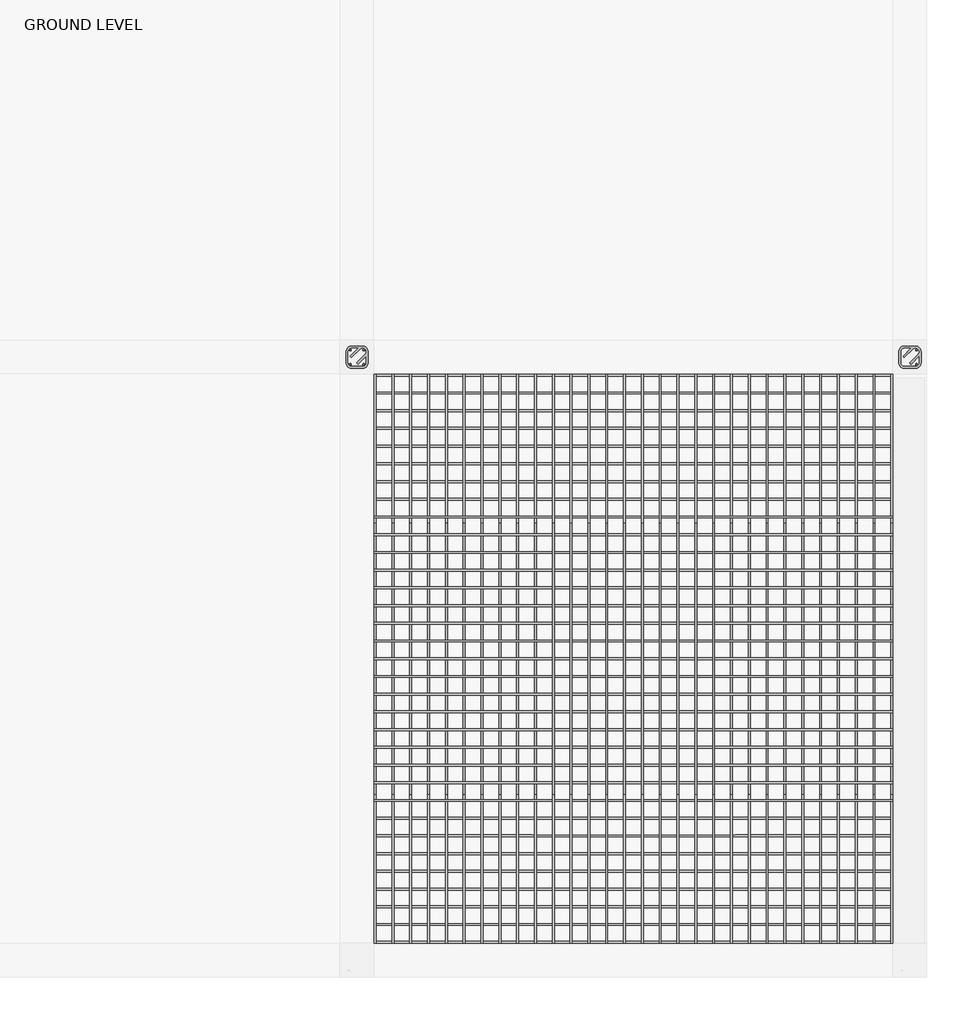
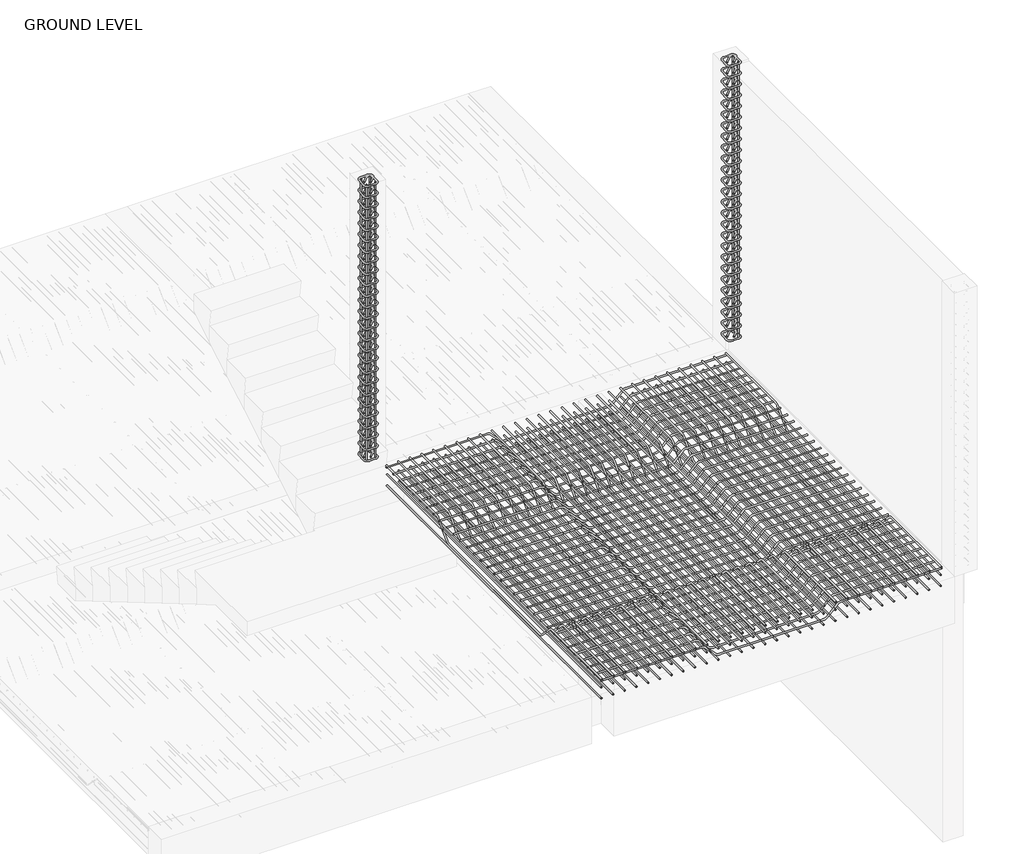
# One storey, part 5 of 8: 9 reinforcing bars.
"""IFC4 building model written with IfcOpenShell, lengths in millimetres."""

from ifc_helpers import new_model, si_unit, point, frame, origin, place, context, project, spatial, polyline, circle_curve, trimmed, segment, composite_curve, source, transform, mapped, element, save
from ifc_brep_helpers import swept_disk

model = new_model("IFC4")

# Units and contexts
model_context = context("Model", 3, world=origin())
ifc_project = project(units=[si_unit("LENGTHUNIT", "METRE", prefix="MILLI")], contexts=[model_context])

# Site, building, storey
site = spatial("IfcSite", under=ifc_project)
building = spatial("IfcBuilding", under=site)
storey = spatial("IfcBuildingStorey", under=building, Name="GROUND LEVEL", Elevation=0.0)

# Reinforcing bars
placement = place(None, origin())
reinforcing_bar_shape = source(origin(), model_context, "Body", "SolidModel", [
    swept_disk(composite_curve([segment(polyline([(-7200.1673382, -353.3525279, -46.35), (-6173.0161368, -353.3525279, -46.35)]), True, "CONTINUOUS"), segment(trimmed(circle_curve(frame((-6173.0161368, -353.3525279, -92.7), z_axis=(0.0, 1.0, 0.0), x_axis=(0.0, 0.0, 46.35)), 46.35), [point((-6173.0161368, -353.3525279, -46.35))], [point((-6140.2417375, -353.3525279, -59.9256007))], True, "CARTESIAN"), True, "CONTINUOUS"), segment(polyline([(-6140.2417375, -353.3525279, -59.9256007), (-6032.3215826, -353.3525279, -167.8457555)]), True, "CONTINUOUS"), segment(trimmed(circle_curve(frame((-5999.5471833, -353.3525279, -135.0713562), z_axis=(0.0, -1.0, 0.0), x_axis=(-32.77439929999946, 0.0, -32.7743993)), 46.35), [point((-6032.3215826, -353.3525279, -167.8457555))], [point((-5999.5471833, -353.3525279, -181.4213562))], True, "CARTESIAN"), True, "CONTINUOUS"), segment(polyline([(-5999.5471833, -353.3525279, -181.4213562), (-4935.6758347, -353.3525279, -181.4213562)]), True, "CONTINUOUS"), segment(trimmed(circle_curve(frame((-4935.6758347, -353.3525279, -135.0713562), z_axis=(0.0, -1.0, 0.0), x_axis=(0.0, 0.0, -46.349999999999994)), 46.35), [point((-4935.6758347, -353.3525279, -181.4213562))], [point((-4902.9014354, -353.3525279, -167.8457555))], True, "CARTESIAN"), True, "CONTINUOUS"), segment(polyline([(-4902.9014354, -353.3525279, -167.8457555), (-4794.9812806, -353.3525279, -59.9256007)]), True, "CONTINUOUS"), segment(trimmed(circle_curve(frame((-4762.2068813, -353.3525279, -92.7), z_axis=(0.0, 1.0, 0.0), x_axis=(-32.77439930000037, 0.0, 32.774399300000006)), 46.35), [point((-4794.9812806, -353.3525279, -59.9256007))], [point((-4762.2068813, -353.3525279, -46.35))], True, "CARTESIAN"), True, "CONTINUOUS"), segment(polyline([(-4762.2068813, -353.3525279, -46.35), (-3735.0556799, -353.3525279, -46.35)]), True, "CONTINUOUS")], self_intersect=False), 6.35),
])
element("IfcReinforcingBar", 1, at=placement, inside=storey, context=model_context, shape_type="MappedRepresentation", body=[
    mapped(reinforcing_bar_shape, transform((0.0, 0.0, 0.0), x_axis=(1.0, 0.0, 0.0), y_axis=(0.0, 1.0, 0.0), z_axis=(0.0, 0.0, 1.0))),
    mapped(reinforcing_bar_shape, transform((0.0, -118.309244, 0.0), x_axis=(1.0, 0.0, 0.0), y_axis=(0.0, 1.0, 0.0), z_axis=(0.0, 0.0, 1.0))),
    mapped(reinforcing_bar_shape, transform((0.0, -236.6184879, 0.0), x_axis=(1.0, 0.0, 0.0), y_axis=(0.0, 1.0, 0.0), z_axis=(0.0, 0.0, 1.0))),
    mapped(reinforcing_bar_shape, transform((0.0, -354.9277319, 0.0), x_axis=(1.0, 0.0, 0.0), y_axis=(0.0, 1.0, 0.0), z_axis=(0.0, 0.0, 1.0))),
    mapped(reinforcing_bar_shape, transform((0.0, -473.2369759, 0.0), x_axis=(1.0, 0.0, 0.0), y_axis=(0.0, 1.0, 0.0), z_axis=(0.0, 0.0, 1.0))),
    mapped(reinforcing_bar_shape, transform((0.0, -591.5462199, 0.0), x_axis=(1.0, 0.0, 0.0), y_axis=(0.0, 1.0, 0.0), z_axis=(0.0, 0.0, 1.0))),
    mapped(reinforcing_bar_shape, transform((0.0, -709.8554638, 0.0), x_axis=(1.0, 0.0, 0.0), y_axis=(0.0, 1.0, 0.0), z_axis=(0.0, 0.0, 1.0))),
    mapped(reinforcing_bar_shape, transform((0.0, -828.1647078, 0.0), x_axis=(1.0, 0.0, 0.0), y_axis=(0.0, 1.0, 0.0), z_axis=(0.0, 0.0, 1.0))),
    mapped(reinforcing_bar_shape, transform((0.0, -946.4739518, 0.0), x_axis=(1.0, 0.0, 0.0), y_axis=(0.0, 1.0, 0.0), z_axis=(0.0, 0.0, 1.0))),
    mapped(reinforcing_bar_shape, transform((0.0, -1064.7831957, 0.0), x_axis=(1.0, 0.0, 0.0), y_axis=(0.0, 1.0, 0.0), z_axis=(0.0, 0.0, 1.0))),
    mapped(reinforcing_bar_shape, transform((0.0, -1183.0924397, 0.0), x_axis=(1.0, 0.0, 0.0), y_axis=(0.0, 1.0, 0.0), z_axis=(0.0, 0.0, 1.0))),
    mapped(reinforcing_bar_shape, transform((0.0, -1301.4016837, 0.0), x_axis=(1.0, 0.0, 0.0), y_axis=(0.0, 1.0, 0.0), z_axis=(0.0, 0.0, 1.0))),
    mapped(reinforcing_bar_shape, transform((0.0, -1419.7109276, 0.0), x_axis=(1.0, 0.0, 0.0), y_axis=(0.0, 1.0, 0.0), z_axis=(0.0, 0.0, 1.0))),
    mapped(reinforcing_bar_shape, transform((0.0, -1538.0201716, 0.0), x_axis=(1.0, 0.0, 0.0), y_axis=(0.0, 1.0, 0.0), z_axis=(0.0, 0.0, 1.0))),
    mapped(reinforcing_bar_shape, transform((0.0, -1656.3294156, 0.0), x_axis=(1.0, 0.0, 0.0), y_axis=(0.0, 1.0, 0.0), z_axis=(0.0, 0.0, 1.0))),
    mapped(reinforcing_bar_shape, transform((0.0, -1774.6386596, 0.0), x_axis=(1.0, 0.0, 0.0), y_axis=(0.0, 1.0, 0.0), z_axis=(0.0, 0.0, 1.0))),
    mapped(reinforcing_bar_shape, transform((0.0, -1892.9479035, 0.0), x_axis=(1.0, 0.0, 0.0), y_axis=(0.0, 1.0, 0.0), z_axis=(0.0, 0.0, 1.0))),
    mapped(reinforcing_bar_shape, transform((0.0, -2011.2571475, 0.0), x_axis=(1.0, 0.0, 0.0), y_axis=(0.0, 1.0, 0.0), z_axis=(0.0, 0.0, 1.0))),
    mapped(reinforcing_bar_shape, transform((0.0, -2129.5663915, 0.0), x_axis=(1.0, 0.0, 0.0), y_axis=(0.0, 1.0, 0.0), z_axis=(0.0, 0.0, 1.0))),
    mapped(reinforcing_bar_shape, transform((0.0, -2247.8756354, 0.0), x_axis=(1.0, 0.0, 0.0), y_axis=(0.0, 1.0, 0.0), z_axis=(0.0, 0.0, 1.0))),
    mapped(reinforcing_bar_shape, transform((0.0, -2366.1848794, 0.0), x_axis=(1.0, 0.0, 0.0), y_axis=(0.0, 1.0, 0.0), z_axis=(0.0, 0.0, 1.0))),
    mapped(reinforcing_bar_shape, transform((0.0, -2484.4941234, 0.0), x_axis=(1.0, 0.0, 0.0), y_axis=(0.0, 1.0, 0.0), z_axis=(0.0, 0.0, 1.0))),
    mapped(reinforcing_bar_shape, transform((0.0, -2602.8033673, 0.0), x_axis=(1.0, 0.0, 0.0), y_axis=(0.0, 1.0, 0.0), z_axis=(0.0, 0.0, 1.0))),
    mapped(reinforcing_bar_shape, transform((0.0, -2721.1126113, 0.0), x_axis=(1.0, 0.0, 0.0), y_axis=(0.0, 1.0, 0.0), z_axis=(0.0, 0.0, 1.0))),
    mapped(reinforcing_bar_shape, transform((0.0, -2839.4218553, 0.0), x_axis=(1.0, 0.0, 0.0), y_axis=(0.0, 1.0, 0.0), z_axis=(0.0, 0.0, 1.0))),
    mapped(reinforcing_bar_shape, transform((0.0, -2957.7310993, 0.0), x_axis=(1.0, 0.0, 0.0), y_axis=(0.0, 1.0, 0.0), z_axis=(0.0, 0.0, 1.0))),
    mapped(reinforcing_bar_shape, transform((0.0, -3076.0403432, 0.0), x_axis=(1.0, 0.0, 0.0), y_axis=(0.0, 1.0, 0.0), z_axis=(0.0, 0.0, 1.0))),
    mapped(reinforcing_bar_shape, transform((0.0, -3194.3495872, 0.0), x_axis=(1.0, 0.0, 0.0), y_axis=(0.0, 1.0, 0.0), z_axis=(0.0, 0.0, 1.0))),
    mapped(reinforcing_bar_shape, transform((0.0, -3312.6588312, 0.0), x_axis=(1.0, 0.0, 0.0), y_axis=(0.0, 1.0, 0.0), z_axis=(0.0, 0.0, 1.0))),
    mapped(reinforcing_bar_shape, transform((0.0, -3430.9680751, 0.0), x_axis=(1.0, 0.0, 0.0), y_axis=(0.0, 1.0, 0.0), z_axis=(0.0, 0.0, 1.0))),
    mapped(reinforcing_bar_shape, transform((0.0, -3549.2773191, 0.0), x_axis=(1.0, 0.0, 0.0), y_axis=(0.0, 1.0, 0.0), z_axis=(0.0, 0.0, 1.0))),
    mapped(reinforcing_bar_shape, transform((0.0, -3667.5865631, 0.0), x_axis=(1.0, 0.0, 0.0), y_axis=(0.0, 1.0, 0.0), z_axis=(0.0, 0.0, 1.0))),
    mapped(reinforcing_bar_shape, transform((0.0, -3785.895807, 0.0), x_axis=(1.0, 0.0, 0.0), y_axis=(0.0, 1.0, 0.0), z_axis=(0.0, 0.0, 1.0))),
])
reinforcing_bar_2_shape = source(origin(), model_context, "Body", "SolidModel", [
    swept_disk(composite_curve([segment(polyline([(-3741.4056799, -347.0025279, -31.8755724), (-3741.4056799, -1227.8037293, -31.8755724)]), True, "CONTINUOUS"), segment(trimmed(circle_curve(frame((-3741.4056799, -1227.8037293, -78.2255724), z_axis=(1.0, 0.0, 0.0), x_axis=(0.0, 0.0, 46.35000000000001)), 46.35), [point((-3741.4056799, -1227.8037293, -31.8755724))], [point((-3741.4056799, -1260.5781286, -45.4511731))], True, "CARTESIAN"), True, "CONTINUOUS"), segment(polyline([(-3741.4056799, -1260.5781286, -45.4511731), (-3741.4056799, -1410.9101229, -195.7831675)]), True, "CONTINUOUS"), segment(trimmed(circle_curve(frame((-3741.4056799, -1443.6845222, -163.0087682), z_axis=(-1.0000000000000002, 0.0, 0.0), x_axis=(0.0, 32.774399299999914, -32.7743993)), 46.35), [point((-3741.4056799, -1410.9101229, -195.7831675))], [point((-3741.4056799, -1443.6845222, -209.3587682))], True, "CARTESIAN"), True, "CONTINUOUS"), segment(polyline([(-3741.4056799, -1443.6845222, -209.3587682), (-3741.4056799, -3048.9163406, -209.3587682)]), True, "CONTINUOUS"), segment(trimmed(circle_curve(frame((-3741.4056799, -3048.9163406, -163.0087682), z_axis=(-1.0, 0.0, 0.0), x_axis=(0.0, 0.0, -46.349999999999994)), 46.35), [point((-3741.4056799, -3048.9163406, -209.3587682))], [point((-3741.4056799, -3081.6907399, -195.7831675))], True, "CARTESIAN"), True, "CONTINUOUS"), segment(polyline([(-3741.4056799, -3081.6907399, -195.7831675), (-3741.4056799, -3232.0227342, -45.4511731)]), True, "CONTINUOUS"), segment(trimmed(circle_curve(frame((-3741.4056799, -3264.7971335, -78.2255724), z_axis=(1.0, 0.0, 0.0), x_axis=(0.0, 32.77439930000037, 32.774399300000006)), 46.35), [point((-3741.4056799, -3232.0227342, -45.4511731))], [point((-3741.4056799, -3264.7971335, -31.8755724))], True, "CARTESIAN"), True, "CONTINUOUS"), segment(polyline([(-3741.4056799, -3264.7971335, -31.8755724), (-3741.4056799, -4145.5983349, -31.8755724)]), True, "CONTINUOUS")], self_intersect=False), 6.35),
])
element("IfcReinforcingBar", 2, at=placement, inside=storey, context=model_context, shape_type="MappedRepresentation", body=[
    mapped(reinforcing_bar_2_shape, transform((0.0, 0.0, 0.0), x_axis=(1.0, 0.0, 0.0), y_axis=(0.0, 1.0, 0.0), z_axis=(0.0, 0.0, 1.0))),
    mapped(reinforcing_bar_2_shape, transform((-119.0486779, 0.0, 0.0), x_axis=(1.0, 0.0, 0.0), y_axis=(0.0, 1.0, 0.0), z_axis=(0.0, 0.0, 1.0))),
    mapped(reinforcing_bar_2_shape, transform((-238.0973557, 0.0, 0.0), x_axis=(1.0, 0.0, 0.0), y_axis=(0.0, 1.0, 0.0), z_axis=(0.0, 0.0, 1.0))),
    mapped(reinforcing_bar_2_shape, transform((-357.1460336, 0.0, 0.0), x_axis=(1.0, 0.0, 0.0), y_axis=(0.0, 1.0, 0.0), z_axis=(0.0, 0.0, 1.0))),
    mapped(reinforcing_bar_2_shape, transform((-476.1947115, 0.0, 0.0), x_axis=(1.0, 0.0, 0.0), y_axis=(0.0, 1.0, 0.0), z_axis=(0.0, 0.0, 1.0))),
    mapped(reinforcing_bar_2_shape, transform((-595.2433894, 0.0, 0.0), x_axis=(1.0, 0.0, 0.0), y_axis=(0.0, 1.0, 0.0), z_axis=(0.0, 0.0, 1.0))),
    mapped(reinforcing_bar_2_shape, transform((-714.2920672, 0.0, 0.0), x_axis=(1.0, 0.0, 0.0), y_axis=(0.0, 1.0, 0.0), z_axis=(0.0, 0.0, 1.0))),
    mapped(reinforcing_bar_2_shape, transform((-833.3407451, 0.0, 0.0), x_axis=(1.0, 0.0, 0.0), y_axis=(0.0, 1.0, 0.0), z_axis=(0.0, 0.0, 1.0))),
    mapped(reinforcing_bar_2_shape, transform((-952.389423, 0.0, 0.0), x_axis=(1.0, 0.0, 0.0), y_axis=(0.0, 1.0, 0.0), z_axis=(0.0, 0.0, 1.0))),
    mapped(reinforcing_bar_2_shape, transform((-1071.4381009, 0.0, 0.0), x_axis=(1.0, 0.0, 0.0), y_axis=(0.0, 1.0, 0.0), z_axis=(0.0, 0.0, 1.0))),
    mapped(reinforcing_bar_2_shape, transform((-1190.4867787, 0.0, 0.0), x_axis=(1.0, 0.0, 0.0), y_axis=(0.0, 1.0, 0.0), z_axis=(0.0, 0.0, 1.0))),
    mapped(reinforcing_bar_2_shape, transform((-1309.5354566, 0.0, 0.0), x_axis=(1.0, 0.0, 0.0), y_axis=(0.0, 1.0, 0.0), z_axis=(0.0, 0.0, 1.0))),
    mapped(reinforcing_bar_2_shape, transform((-1428.5841345, 0.0, 0.0), x_axis=(1.0, 0.0, 0.0), y_axis=(0.0, 1.0, 0.0), z_axis=(0.0, 0.0, 1.0))),
    mapped(reinforcing_bar_2_shape, transform((-1547.6328123, 0.0, 0.0), x_axis=(1.0, 0.0, 0.0), y_axis=(0.0, 1.0, 0.0), z_axis=(0.0, 0.0, 1.0))),
    mapped(reinforcing_bar_2_shape, transform((-1666.6814902, 0.0, 0.0), x_axis=(1.0, 0.0, 0.0), y_axis=(0.0, 1.0, 0.0), z_axis=(0.0, 0.0, 1.0))),
    mapped(reinforcing_bar_2_shape, transform((-1785.7301681, 0.0, 0.0), x_axis=(1.0, 0.0, 0.0), y_axis=(0.0, 1.0, 0.0), z_axis=(0.0, 0.0, 1.0))),
    mapped(reinforcing_bar_2_shape, transform((-1904.778846, 0.0, 0.0), x_axis=(1.0, 0.0, 0.0), y_axis=(0.0, 1.0, 0.0), z_axis=(0.0, 0.0, 1.0))),
    mapped(reinforcing_bar_2_shape, transform((-2023.8275238, 0.0, 0.0), x_axis=(1.0, 0.0, 0.0), y_axis=(0.0, 1.0, 0.0), z_axis=(0.0, 0.0, 1.0))),
    mapped(reinforcing_bar_2_shape, transform((-2142.8762017, 0.0, 0.0), x_axis=(1.0, 0.0, 0.0), y_axis=(0.0, 1.0, 0.0), z_axis=(0.0, 0.0, 1.0))),
    mapped(reinforcing_bar_2_shape, transform((-2261.9248796, 0.0, 0.0), x_axis=(1.0, 0.0, 0.0), y_axis=(0.0, 1.0, 0.0), z_axis=(0.0, 0.0, 1.0))),
    mapped(reinforcing_bar_2_shape, transform((-2380.9735574, 0.0, 0.0), x_axis=(1.0, 0.0, 0.0), y_axis=(0.0, 1.0, 0.0), z_axis=(0.0, 0.0, 1.0))),
    mapped(reinforcing_bar_2_shape, transform((-2500.0222353, 0.0, 0.0), x_axis=(1.0, 0.0, 0.0), y_axis=(0.0, 1.0, 0.0), z_axis=(0.0, 0.0, 1.0))),
    mapped(reinforcing_bar_2_shape, transform((-2619.0709132, 0.0, 0.0), x_axis=(1.0, 0.0, 0.0), y_axis=(0.0, 1.0, 0.0), z_axis=(0.0, 0.0, 1.0))),
    mapped(reinforcing_bar_2_shape, transform((-2738.1195911, 0.0, 0.0), x_axis=(1.0, 0.0, 0.0), y_axis=(0.0, 1.0, 0.0), z_axis=(0.0, 0.0, 1.0))),
    mapped(reinforcing_bar_2_shape, transform((-2857.1682689, 0.0, 0.0), x_axis=(1.0, 0.0, 0.0), y_axis=(0.0, 1.0, 0.0), z_axis=(0.0, 0.0, 1.0))),
    mapped(reinforcing_bar_2_shape, transform((-2976.2169468, 0.0, 0.0), x_axis=(1.0, 0.0, 0.0), y_axis=(0.0, 1.0, 0.0), z_axis=(0.0, 0.0, 1.0))),
    mapped(reinforcing_bar_2_shape, transform((-3095.2656247, 0.0, 0.0), x_axis=(1.0, 0.0, 0.0), y_axis=(0.0, 1.0, 0.0), z_axis=(0.0, 0.0, 1.0))),
    mapped(reinforcing_bar_2_shape, transform((-3214.3143026, 0.0, 0.0), x_axis=(1.0, 0.0, 0.0), y_axis=(0.0, 1.0, 0.0), z_axis=(0.0, 0.0, 1.0))),
    mapped(reinforcing_bar_2_shape, transform((-3333.3629804, 0.0, 0.0), x_axis=(1.0, 0.0, 0.0), y_axis=(0.0, 1.0, 0.0), z_axis=(0.0, 0.0, 1.0))),
    mapped(reinforcing_bar_2_shape, transform((-3452.4116583, 0.0, 0.0), x_axis=(1.0, 0.0, 0.0), y_axis=(0.0, 1.0, 0.0), z_axis=(0.0, 0.0, 1.0))),
])
reinforcing_bar_3_shape = source(origin(), model_context, "Body", "SolidModel", [
    swept_disk(composite_curve([segment(polyline([(-3741.4056799, -4134.0810507, -240.830741), (-3741.4056799, -358.1289151, -240.830741)]), True, "CONTINUOUS")], self_intersect=False), 6.35),
])
element("IfcReinforcingBar", 3, at=placement, inside=storey, context=model_context, shape_type="MappedRepresentation", body=[
    mapped(reinforcing_bar_3_shape, transform((0.0, 0.0, 0.0), x_axis=(1.0, 0.0, 0.0), y_axis=(0.0, 1.0, 0.0), z_axis=(0.0, 0.0, 1.0))),
    mapped(reinforcing_bar_3_shape, transform((-119.0486779, 0.0, 0.0), x_axis=(1.0, 0.0, 0.0), y_axis=(0.0, 1.0, 0.0), z_axis=(0.0, 0.0, 1.0))),
    mapped(reinforcing_bar_3_shape, transform((-238.0973557, 0.0, 0.0), x_axis=(1.0, 0.0, 0.0), y_axis=(0.0, 1.0, 0.0), z_axis=(0.0, 0.0, 1.0))),
    mapped(reinforcing_bar_3_shape, transform((-357.1460336, 0.0, 0.0), x_axis=(1.0, 0.0, 0.0), y_axis=(0.0, 1.0, 0.0), z_axis=(0.0, 0.0, 1.0))),
    mapped(reinforcing_bar_3_shape, transform((-476.1947115, 0.0, 0.0), x_axis=(1.0, 0.0, 0.0), y_axis=(0.0, 1.0, 0.0), z_axis=(0.0, 0.0, 1.0))),
    mapped(reinforcing_bar_3_shape, transform((-595.2433894, 0.0, 0.0), x_axis=(1.0, 0.0, 0.0), y_axis=(0.0, 1.0, 0.0), z_axis=(0.0, 0.0, 1.0))),
    mapped(reinforcing_bar_3_shape, transform((-714.2920672, 0.0, 0.0), x_axis=(1.0, 0.0, 0.0), y_axis=(0.0, 1.0, 0.0), z_axis=(0.0, 0.0, 1.0))),
    mapped(reinforcing_bar_3_shape, transform((-833.3407451, 0.0, 0.0), x_axis=(1.0, 0.0, 0.0), y_axis=(0.0, 1.0, 0.0), z_axis=(0.0, 0.0, 1.0))),
    mapped(reinforcing_bar_3_shape, transform((-952.389423, 0.0, 0.0), x_axis=(1.0, 0.0, 0.0), y_axis=(0.0, 1.0, 0.0), z_axis=(0.0, 0.0, 1.0))),
    mapped(reinforcing_bar_3_shape, transform((-1071.4381009, 0.0, 0.0), x_axis=(1.0, 0.0, 0.0), y_axis=(0.0, 1.0, 0.0), z_axis=(0.0, 0.0, 1.0))),
    mapped(reinforcing_bar_3_shape, transform((-1190.4867787, 0.0, 0.0), x_axis=(1.0, 0.0, 0.0), y_axis=(0.0, 1.0, 0.0), z_axis=(0.0, 0.0, 1.0))),
    mapped(reinforcing_bar_3_shape, transform((-1309.5354566, 0.0, 0.0), x_axis=(1.0, 0.0, 0.0), y_axis=(0.0, 1.0, 0.0), z_axis=(0.0, 0.0, 1.0))),
    mapped(reinforcing_bar_3_shape, transform((-1428.5841345, 0.0, 0.0), x_axis=(1.0, 0.0, 0.0), y_axis=(0.0, 1.0, 0.0), z_axis=(0.0, 0.0, 1.0))),
    mapped(reinforcing_bar_3_shape, transform((-1547.6328123, 0.0, 0.0), x_axis=(1.0, 0.0, 0.0), y_axis=(0.0, 1.0, 0.0), z_axis=(0.0, 0.0, 1.0))),
    mapped(reinforcing_bar_3_shape, transform((-1666.6814902, 0.0, 0.0), x_axis=(1.0, 0.0, 0.0), y_axis=(0.0, 1.0, 0.0), z_axis=(0.0, 0.0, 1.0))),
    mapped(reinforcing_bar_3_shape, transform((-1785.7301681, 0.0, 0.0), x_axis=(1.0, 0.0, 0.0), y_axis=(0.0, 1.0, 0.0), z_axis=(0.0, 0.0, 1.0))),
    mapped(reinforcing_bar_3_shape, transform((-1904.778846, 0.0, 0.0), x_axis=(1.0, 0.0, 0.0), y_axis=(0.0, 1.0, 0.0), z_axis=(0.0, 0.0, 1.0))),
    mapped(reinforcing_bar_3_shape, transform((-2023.8275238, 0.0, 0.0), x_axis=(1.0, 0.0, 0.0), y_axis=(0.0, 1.0, 0.0), z_axis=(0.0, 0.0, 1.0))),
    mapped(reinforcing_bar_3_shape, transform((-2142.8762017, 0.0, 0.0), x_axis=(1.0, 0.0, 0.0), y_axis=(0.0, 1.0, 0.0), z_axis=(0.0, 0.0, 1.0))),
    mapped(reinforcing_bar_3_shape, transform((-2261.9248796, 0.0, 0.0), x_axis=(1.0, 0.0, 0.0), y_axis=(0.0, 1.0, 0.0), z_axis=(0.0, 0.0, 1.0))),
    mapped(reinforcing_bar_3_shape, transform((-2380.9735574, 0.0, 0.0), x_axis=(1.0, 0.0, 0.0), y_axis=(0.0, 1.0, 0.0), z_axis=(0.0, 0.0, 1.0))),
    mapped(reinforcing_bar_3_shape, transform((-2500.0222353, 0.0, 0.0), x_axis=(1.0, 0.0, 0.0), y_axis=(0.0, 1.0, 0.0), z_axis=(0.0, 0.0, 1.0))),
    mapped(reinforcing_bar_3_shape, transform((-2619.0709132, 0.0, 0.0), x_axis=(1.0, 0.0, 0.0), y_axis=(0.0, 1.0, 0.0), z_axis=(0.0, 0.0, 1.0))),
    mapped(reinforcing_bar_3_shape, transform((-2738.1195911, 0.0, 0.0), x_axis=(1.0, 0.0, 0.0), y_axis=(0.0, 1.0, 0.0), z_axis=(0.0, 0.0, 1.0))),
    mapped(reinforcing_bar_3_shape, transform((-2857.1682689, 0.0, 0.0), x_axis=(1.0, 0.0, 0.0), y_axis=(0.0, 1.0, 0.0), z_axis=(0.0, 0.0, 1.0))),
    mapped(reinforcing_bar_3_shape, transform((-2976.2169468, 0.0, 0.0), x_axis=(1.0, 0.0, 0.0), y_axis=(0.0, 1.0, 0.0), z_axis=(0.0, 0.0, 1.0))),
    mapped(reinforcing_bar_3_shape, transform((-3095.2656247, 0.0, 0.0), x_axis=(1.0, 0.0, 0.0), y_axis=(0.0, 1.0, 0.0), z_axis=(0.0, 0.0, 1.0))),
    mapped(reinforcing_bar_3_shape, transform((-3214.3143026, 0.0, 0.0), x_axis=(1.0, 0.0, 0.0), y_axis=(0.0, 1.0, 0.0), z_axis=(0.0, 0.0, 1.0))),
    mapped(reinforcing_bar_3_shape, transform((-3333.3629804, 0.0, 0.0), x_axis=(1.0, 0.0, 0.0), y_axis=(0.0, 1.0, 0.0), z_axis=(0.0, 0.0, 1.0))),
    mapped(reinforcing_bar_3_shape, transform((-3452.4116583, 0.0, 0.0), x_axis=(1.0, 0.0, 0.0), y_axis=(0.0, 1.0, 0.0), z_axis=(0.0, 0.0, 1.0))),
])
reinforcing_bar_4_shape = source(origin(), model_context, "Body", "SolidModel", [
    swept_disk(composite_curve([segment(polyline([(-3741.4056799, -4134.0810507, -120.830741), (-3741.4056799, -358.1289151, -120.830741)]), True, "CONTINUOUS")], self_intersect=False), 6.35),
])
element("IfcReinforcingBar", 4, at=placement, inside=storey, context=model_context, shape_type="MappedRepresentation", body=[
    mapped(reinforcing_bar_4_shape, transform((0.0, 0.0, 0.0), x_axis=(1.0, 0.0, 0.0), y_axis=(0.0, 1.0, 0.0), z_axis=(0.0, 0.0, 1.0))),
    mapped(reinforcing_bar_4_shape, transform((-119.0486779, 0.0, 0.0), x_axis=(1.0, 0.0, 0.0), y_axis=(0.0, 1.0, 0.0), z_axis=(0.0, 0.0, 1.0))),
    mapped(reinforcing_bar_4_shape, transform((-238.0973557, 0.0, 0.0), x_axis=(1.0, 0.0, 0.0), y_axis=(0.0, 1.0, 0.0), z_axis=(0.0, 0.0, 1.0))),
    mapped(reinforcing_bar_4_shape, transform((-357.1460336, 0.0, 0.0), x_axis=(1.0, 0.0, 0.0), y_axis=(0.0, 1.0, 0.0), z_axis=(0.0, 0.0, 1.0))),
    mapped(reinforcing_bar_4_shape, transform((-476.1947115, 0.0, 0.0), x_axis=(1.0, 0.0, 0.0), y_axis=(0.0, 1.0, 0.0), z_axis=(0.0, 0.0, 1.0))),
    mapped(reinforcing_bar_4_shape, transform((-595.2433894, 0.0, 0.0), x_axis=(1.0, 0.0, 0.0), y_axis=(0.0, 1.0, 0.0), z_axis=(0.0, 0.0, 1.0))),
    mapped(reinforcing_bar_4_shape, transform((-714.2920672, 0.0, 0.0), x_axis=(1.0, 0.0, 0.0), y_axis=(0.0, 1.0, 0.0), z_axis=(0.0, 0.0, 1.0))),
    mapped(reinforcing_bar_4_shape, transform((-833.3407451, 0.0, 0.0), x_axis=(1.0, 0.0, 0.0), y_axis=(0.0, 1.0, 0.0), z_axis=(0.0, 0.0, 1.0))),
    mapped(reinforcing_bar_4_shape, transform((-952.389423, 0.0, 0.0), x_axis=(1.0, 0.0, 0.0), y_axis=(0.0, 1.0, 0.0), z_axis=(0.0, 0.0, 1.0))),
    mapped(reinforcing_bar_4_shape, transform((-1071.4381009, 0.0, 0.0), x_axis=(1.0, 0.0, 0.0), y_axis=(0.0, 1.0, 0.0), z_axis=(0.0, 0.0, 1.0))),
    mapped(reinforcing_bar_4_shape, transform((-1190.4867787, 0.0, 0.0), x_axis=(1.0, 0.0, 0.0), y_axis=(0.0, 1.0, 0.0), z_axis=(0.0, 0.0, 1.0))),
    mapped(reinforcing_bar_4_shape, transform((-1309.5354566, 0.0, 0.0), x_axis=(1.0, 0.0, 0.0), y_axis=(0.0, 1.0, 0.0), z_axis=(0.0, 0.0, 1.0))),
    mapped(reinforcing_bar_4_shape, transform((-1428.5841345, 0.0, 0.0), x_axis=(1.0, 0.0, 0.0), y_axis=(0.0, 1.0, 0.0), z_axis=(0.0, 0.0, 1.0))),
    mapped(reinforcing_bar_4_shape, transform((-1547.6328123, 0.0, 0.0), x_axis=(1.0, 0.0, 0.0), y_axis=(0.0, 1.0, 0.0), z_axis=(0.0, 0.0, 1.0))),
    mapped(reinforcing_bar_4_shape, transform((-1666.6814902, 0.0, 0.0), x_axis=(1.0, 0.0, 0.0), y_axis=(0.0, 1.0, 0.0), z_axis=(0.0, 0.0, 1.0))),
    mapped(reinforcing_bar_4_shape, transform((-1785.7301681, 0.0, 0.0), x_axis=(1.0, 0.0, 0.0), y_axis=(0.0, 1.0, 0.0), z_axis=(0.0, 0.0, 1.0))),
    mapped(reinforcing_bar_4_shape, transform((-1904.778846, 0.0, 0.0), x_axis=(1.0, 0.0, 0.0), y_axis=(0.0, 1.0, 0.0), z_axis=(0.0, 0.0, 1.0))),
    mapped(reinforcing_bar_4_shape, transform((-2023.8275238, 0.0, 0.0), x_axis=(1.0, 0.0, 0.0), y_axis=(0.0, 1.0, 0.0), z_axis=(0.0, 0.0, 1.0))),
    mapped(reinforcing_bar_4_shape, transform((-2142.8762017, 0.0, 0.0), x_axis=(1.0, 0.0, 0.0), y_axis=(0.0, 1.0, 0.0), z_axis=(0.0, 0.0, 1.0))),
    mapped(reinforcing_bar_4_shape, transform((-2261.9248796, 0.0, 0.0), x_axis=(1.0, 0.0, 0.0), y_axis=(0.0, 1.0, 0.0), z_axis=(0.0, 0.0, 1.0))),
    mapped(reinforcing_bar_4_shape, transform((-2380.9735574, 0.0, 0.0), x_axis=(1.0, 0.0, 0.0), y_axis=(0.0, 1.0, 0.0), z_axis=(0.0, 0.0, 1.0))),
    mapped(reinforcing_bar_4_shape, transform((-2500.0222353, 0.0, 0.0), x_axis=(1.0, 0.0, 0.0), y_axis=(0.0, 1.0, 0.0), z_axis=(0.0, 0.0, 1.0))),
    mapped(reinforcing_bar_4_shape, transform((-2619.0709132, 0.0, 0.0), x_axis=(1.0, 0.0, 0.0), y_axis=(0.0, 1.0, 0.0), z_axis=(0.0, 0.0, 1.0))),
    mapped(reinforcing_bar_4_shape, transform((-2738.1195911, 0.0, 0.0), x_axis=(1.0, 0.0, 0.0), y_axis=(0.0, 1.0, 0.0), z_axis=(0.0, 0.0, 1.0))),
    mapped(reinforcing_bar_4_shape, transform((-2857.1682689, 0.0, 0.0), x_axis=(1.0, 0.0, 0.0), y_axis=(0.0, 1.0, 0.0), z_axis=(0.0, 0.0, 1.0))),
    mapped(reinforcing_bar_4_shape, transform((-2976.2169468, 0.0, 0.0), x_axis=(1.0, 0.0, 0.0), y_axis=(0.0, 1.0, 0.0), z_axis=(0.0, 0.0, 1.0))),
    mapped(reinforcing_bar_4_shape, transform((-3095.2656247, 0.0, 0.0), x_axis=(1.0, 0.0, 0.0), y_axis=(0.0, 1.0, 0.0), z_axis=(0.0, 0.0, 1.0))),
    mapped(reinforcing_bar_4_shape, transform((-3214.3143026, 0.0, 0.0), x_axis=(1.0, 0.0, 0.0), y_axis=(0.0, 1.0, 0.0), z_axis=(0.0, 0.0, 1.0))),
    mapped(reinforcing_bar_4_shape, transform((-3333.3629804, 0.0, 0.0), x_axis=(1.0, 0.0, 0.0), y_axis=(0.0, 1.0, 0.0), z_axis=(0.0, 0.0, 1.0))),
    mapped(reinforcing_bar_4_shape, transform((-3452.4116583, 0.0, 0.0), x_axis=(1.0, 0.0, 0.0), y_axis=(0.0, 1.0, 0.0), z_axis=(0.0, 0.0, 1.0))),
])
reinforcing_bar_5_shape = source(origin(), model_context, "Body", "SolidModel", [
    swept_disk(composite_curve([segment(polyline([(-3576.0006936, -183.9048321, 3008.0), (-3576.0006936, -183.9048321, 40.0)]), True, "CONTINUOUS")], self_intersect=False), 6.35),
])
element("IfcReinforcingBar", 5, at=placement, inside=storey, context=model_context, shape_type="MappedRepresentation", body=[
    mapped(reinforcing_bar_5_shape, transform((0.0, 0.0, 0.0), x_axis=(1.0, 0.0, 0.0), y_axis=(0.0, 1.0, 0.0), z_axis=(0.0, 0.0, 1.0))),
    mapped(reinforcing_bar_5_shape, transform((0.0, -96.9916148, 0.0), x_axis=(1.0, 0.0, 0.0), y_axis=(0.0, 1.0, 0.0), z_axis=(0.0, 0.0, 1.0))),
])
reinforcing_bar_6_shape = source(origin(), model_context, "Body", "SolidModel", [
    swept_disk(composite_curve([segment(polyline([(-3662.0670404, -229.6782932, 3001.65), (-3606.3234775, -173.9347303, 3001.65)]), True, "CONTINUOUS"), segment(trimmed(circle_curve(frame((-3584.1556799, -196.1025279, 3001.65), z_axis=(0.0, 0.0, -1.0), x_axis=(-22.167797600000085, 22.1677976, 0.0)), 31.35), [point((-3606.3234775, -173.9347303, 3001.65))], [point((-3552.8056799, -196.1025279, 3001.65))], True, "CARTESIAN"), True, "CONTINUOUS"), segment(polyline([(-3552.8056799, -196.1025279, 3001.65), (-3552.8056799, -269.3025279, 3001.65)]), True, "CONTINUOUS"), segment(trimmed(circle_curve(frame((-3584.1556799, -269.3025279, 3001.65), z_axis=(0.0, 0.0, -1.0), x_axis=(31.34999999999991, 0.0, 0.0)), 31.35), [point((-3552.8056799, -269.3025279, 3001.65))], [point((-3584.1556799, -300.6525279, 3001.65))], True, "CARTESIAN"), True, "CONTINUOUS"), segment(polyline([(-3584.1556799, -300.6525279, 3001.65), (-3657.3556799, -300.6525279, 3001.65)]), True, "CONTINUOUS"), segment(trimmed(circle_curve(frame((-3657.3556799, -269.4385291, 3004.5669815), z_axis=(0.0, 0.09304566152621355, -0.9956618426308951), x_axis=(0.0, -31.213998800000013, -2.91698150000002)), 31.35), [point((-3657.3556799, -300.6525279, 3001.65))], [point((-3688.7056799, -269.4385291, 3004.5669815))], True, "CARTESIAN"), True, "CONTINUOUS"), segment(polyline([(-3688.7056799, -269.4385291, 3004.5669815), (-3688.7056799, -195.9665266, 3011.4330185)]), True, "CONTINUOUS"), segment(trimmed(circle_curve(frame((-3657.3556799, -195.9665266, 3011.4330185), z_axis=(0.0, 0.09304566152621355, -0.9956618426308951), x_axis=(-31.350000000000364, 0.0, 0.0)), 31.35), [point((-3688.7056799, -195.9665266, 3011.4330185))], [point((-3657.3556799, -164.7525279, 3014.35))], True, "CARTESIAN"), True, "CONTINUOUS"), segment(polyline([(-3657.3556799, -164.7525279, 3014.35), (-3584.1556799, -164.7525279, 3014.35)]), True, "CONTINUOUS"), segment(trimmed(circle_curve(frame((-3584.1556799, -196.1025279, 3014.35), z_axis=(0.0, 0.0, -1.0), x_axis=(0.0, 31.350000000000023, 0.0)), 31.35), [point((-3584.1556799, -164.7525279, 3014.35))], [point((-3561.9878823, -218.2703255, 3014.35))], True, "CARTESIAN"), True, "CONTINUOUS"), segment(polyline([(-3561.9878823, -218.2703255, 3014.35), (-3617.7314452, -274.0138884, 3014.35)]), True, "CONTINUOUS")], self_intersect=False), 6.35),
])
element("IfcReinforcingBar", 6, at=placement, inside=storey, context=model_context, shape_type="MappedRepresentation", body=[
    mapped(reinforcing_bar_6_shape, transform((0.0, 0.0, 0.0), x_axis=(1.0, 0.0, 0.0), y_axis=(0.0, 1.0, 0.0), z_axis=(0.0, 0.0, 1.0))),
    mapped(reinforcing_bar_6_shape, transform((0.0, 0.0, -118.212), x_axis=(1.0, 0.0, 0.0), y_axis=(0.0, 1.0, 0.0), z_axis=(0.0, 0.0, 1.0))),
    mapped(reinforcing_bar_6_shape, transform((0.0, 0.0, -236.424), x_axis=(1.0, 0.0, 0.0), y_axis=(0.0, 1.0, 0.0), z_axis=(0.0, 0.0, 1.0))),
    mapped(reinforcing_bar_6_shape, transform((0.0, 0.0, -354.636), x_axis=(1.0, 0.0, 0.0), y_axis=(0.0, 1.0, 0.0), z_axis=(0.0, 0.0, 1.0))),
    mapped(reinforcing_bar_6_shape, transform((0.0, 0.0, -472.848), x_axis=(1.0, 0.0, 0.0), y_axis=(0.0, 1.0, 0.0), z_axis=(0.0, 0.0, 1.0))),
    mapped(reinforcing_bar_6_shape, transform((0.0, 0.0, -591.06), x_axis=(1.0, 0.0, 0.0), y_axis=(0.0, 1.0, 0.0), z_axis=(0.0, 0.0, 1.0))),
    mapped(reinforcing_bar_6_shape, transform((0.0, 0.0, -709.272), x_axis=(1.0, 0.0, 0.0), y_axis=(0.0, 1.0, 0.0), z_axis=(0.0, 0.0, 1.0))),
    mapped(reinforcing_bar_6_shape, transform((0.0, 0.0, -827.484), x_axis=(1.0, 0.0, 0.0), y_axis=(0.0, 1.0, 0.0), z_axis=(0.0, 0.0, 1.0))),
    mapped(reinforcing_bar_6_shape, transform((0.0, 0.0, -945.696), x_axis=(1.0, 0.0, 0.0), y_axis=(0.0, 1.0, 0.0), z_axis=(0.0, 0.0, 1.0))),
    mapped(reinforcing_bar_6_shape, transform((0.0, 0.0, -1063.908), x_axis=(1.0, 0.0, 0.0), y_axis=(0.0, 1.0, 0.0), z_axis=(0.0, 0.0, 1.0))),
    mapped(reinforcing_bar_6_shape, transform((0.0, 0.0, -1182.12), x_axis=(1.0, 0.0, 0.0), y_axis=(0.0, 1.0, 0.0), z_axis=(0.0, 0.0, 1.0))),
    mapped(reinforcing_bar_6_shape, transform((0.0, 0.0, -1300.332), x_axis=(1.0, 0.0, 0.0), y_axis=(0.0, 1.0, 0.0), z_axis=(0.0, 0.0, 1.0))),
    mapped(reinforcing_bar_6_shape, transform((0.0, 0.0, -1418.544), x_axis=(1.0, 0.0, 0.0), y_axis=(0.0, 1.0, 0.0), z_axis=(0.0, 0.0, 1.0))),
    mapped(reinforcing_bar_6_shape, transform((0.0, 0.0, -1536.756), x_axis=(1.0, 0.0, 0.0), y_axis=(0.0, 1.0, 0.0), z_axis=(0.0, 0.0, 1.0))),
    mapped(reinforcing_bar_6_shape, transform((0.0, 0.0, -1654.968), x_axis=(1.0, 0.0, 0.0), y_axis=(0.0, 1.0, 0.0), z_axis=(0.0, 0.0, 1.0))),
    mapped(reinforcing_bar_6_shape, transform((0.0, 0.0, -1773.18), x_axis=(1.0, 0.0, 0.0), y_axis=(0.0, 1.0, 0.0), z_axis=(0.0, 0.0, 1.0))),
    mapped(reinforcing_bar_6_shape, transform((0.0, 0.0, -1891.392), x_axis=(1.0, 0.0, 0.0), y_axis=(0.0, 1.0, 0.0), z_axis=(0.0, 0.0, 1.0))),
    mapped(reinforcing_bar_6_shape, transform((0.0, 0.0, -2009.604), x_axis=(1.0, 0.0, 0.0), y_axis=(0.0, 1.0, 0.0), z_axis=(0.0, 0.0, 1.0))),
    mapped(reinforcing_bar_6_shape, transform((0.0, 0.0, -2127.816), x_axis=(1.0, 0.0, 0.0), y_axis=(0.0, 1.0, 0.0), z_axis=(0.0, 0.0, 1.0))),
    mapped(reinforcing_bar_6_shape, transform((0.0, 0.0, -2246.028), x_axis=(1.0, 0.0, 0.0), y_axis=(0.0, 1.0, 0.0), z_axis=(0.0, 0.0, 1.0))),
    mapped(reinforcing_bar_6_shape, transform((0.0, 0.0, -2364.24), x_axis=(1.0, 0.0, 0.0), y_axis=(0.0, 1.0, 0.0), z_axis=(0.0, 0.0, 1.0))),
    mapped(reinforcing_bar_6_shape, transform((0.0, 0.0, -2482.452), x_axis=(1.0, 0.0, 0.0), y_axis=(0.0, 1.0, 0.0), z_axis=(0.0, 0.0, 1.0))),
    mapped(reinforcing_bar_6_shape, transform((0.0, 0.0, -2600.664), x_axis=(1.0, 0.0, 0.0), y_axis=(0.0, 1.0, 0.0), z_axis=(0.0, 0.0, 1.0))),
    mapped(reinforcing_bar_6_shape, transform((0.0, 0.0, -2718.876), x_axis=(1.0, 0.0, 0.0), y_axis=(0.0, 1.0, 0.0), z_axis=(0.0, 0.0, 1.0))),
    mapped(reinforcing_bar_6_shape, transform((0.0, 0.0, -2837.088), x_axis=(1.0, 0.0, 0.0), y_axis=(0.0, 1.0, 0.0), z_axis=(0.0, 0.0, 1.0))),
    mapped(reinforcing_bar_6_shape, transform((0.0, 0.0, -2955.3), x_axis=(1.0, 0.0, 0.0), y_axis=(0.0, 1.0, 0.0), z_axis=(0.0, 0.0, 1.0))),
])
reinforcing_bar_7_shape = source(origin(), model_context, "Body", "SolidModel", [
    swept_disk(composite_curve([segment(polyline([(-7269.7123519, -183.9048321, 3008.0), (-7269.7123519, -183.9048321, 40.0)]), True, "CONTINUOUS")], self_intersect=False), 6.35),
])
element("IfcReinforcingBar", 7, at=placement, inside=storey, context=model_context, shape_type="MappedRepresentation", body=[
    mapped(reinforcing_bar_7_shape, transform((0.0, 0.0, 0.0), x_axis=(1.0, 0.0, 0.0), y_axis=(0.0, 1.0, 0.0), z_axis=(0.0, 0.0, 1.0))),
    mapped(reinforcing_bar_7_shape, transform((0.0, -96.9916148, 0.0), x_axis=(1.0, 0.0, 0.0), y_axis=(0.0, 1.0, 0.0), z_axis=(0.0, 0.0, 1.0))),
])
reinforcing_bar_8_shape = source(origin(), model_context, "Body", "SolidModel", [
    swept_disk(composite_curve([segment(polyline([(-7355.7786987, -229.6782932, 3001.65), (-7300.0351358, -173.9347303, 3001.65)]), True, "CONTINUOUS"), segment(trimmed(circle_curve(frame((-7277.8673382, -196.1025279, 3001.65), z_axis=(0.0, 0.0, -1.0), x_axis=(-22.167797600000085, 22.1677976, 0.0)), 31.35), [point((-7300.0351358, -173.9347303, 3001.65))], [point((-7246.5173382, -196.1025279, 3001.65))], True, "CARTESIAN"), True, "CONTINUOUS"), segment(polyline([(-7246.5173382, -196.1025279, 3001.65), (-7246.5173382, -269.3025279, 3001.65)]), True, "CONTINUOUS"), segment(trimmed(circle_curve(frame((-7277.8673382, -269.3025279, 3001.65), z_axis=(0.0, 0.0, -1.0), x_axis=(31.349999999999454, 0.0, 0.0)), 31.35), [point((-7246.5173382, -269.3025279, 3001.65))], [point((-7277.8673382, -300.6525279, 3001.65))], True, "CARTESIAN"), True, "CONTINUOUS"), segment(polyline([(-7277.8673382, -300.6525279, 3001.65), (-7351.0673382, -300.6525279, 3001.65)]), True, "CONTINUOUS"), segment(trimmed(circle_curve(frame((-7351.0673382, -269.4385291, 3004.5669815), z_axis=(0.0, 0.09304566152621355, -0.9956618426308951), x_axis=(0.0, -31.213998800000013, -2.91698150000002)), 31.35), [point((-7351.0673382, -300.6525279, 3001.65))], [point((-7382.4173382, -269.4385291, 3004.5669815))], True, "CARTESIAN"), True, "CONTINUOUS"), segment(polyline([(-7382.4173382, -269.4385291, 3004.5669815), (-7382.4173382, -195.9665266, 3011.4330185)]), True, "CONTINUOUS"), segment(trimmed(circle_curve(frame((-7351.0673382, -195.9665266, 3011.4330185), z_axis=(0.0, 0.09304566152621355, -0.9956618426308951), x_axis=(-31.349999999999454, 0.0, 0.0)), 31.35), [point((-7382.4173382, -195.9665266, 3011.4330185))], [point((-7351.0673382, -164.7525279, 3014.35))], True, "CARTESIAN"), True, "CONTINUOUS"), segment(polyline([(-7351.0673382, -164.7525279, 3014.35), (-7277.8673382, -164.7525279, 3014.35)]), True, "CONTINUOUS"), segment(trimmed(circle_curve(frame((-7277.8673382, -196.1025279, 3014.35), z_axis=(0.0, 0.0, -1.0), x_axis=(0.0, 31.350000000000023, 0.0)), 31.35), [point((-7277.8673382, -164.7525279, 3014.35))], [point((-7255.6995406, -218.2703255, 3014.35))], True, "CARTESIAN"), True, "CONTINUOUS"), segment(polyline([(-7255.6995406, -218.2703255, 3014.35), (-7311.4431035, -274.0138884, 3014.35)]), True, "CONTINUOUS")], self_intersect=False), 6.35),
])
element("IfcReinforcingBar", 8, at=placement, inside=storey, context=model_context, shape_type="MappedRepresentation", body=[
    mapped(reinforcing_bar_8_shape, transform((0.0, 0.0, 0.0), x_axis=(1.0, 0.0, 0.0), y_axis=(0.0, 1.0, 0.0), z_axis=(0.0, 0.0, 1.0))),
    mapped(reinforcing_bar_8_shape, transform((0.0, 0.0, -118.212), x_axis=(1.0, 0.0, 0.0), y_axis=(0.0, 1.0, 0.0), z_axis=(0.0, 0.0, 1.0))),
    mapped(reinforcing_bar_8_shape, transform((0.0, 0.0, -236.424), x_axis=(1.0, 0.0, 0.0), y_axis=(0.0, 1.0, 0.0), z_axis=(0.0, 0.0, 1.0))),
    mapped(reinforcing_bar_8_shape, transform((0.0, 0.0, -354.636), x_axis=(1.0, 0.0, 0.0), y_axis=(0.0, 1.0, 0.0), z_axis=(0.0, 0.0, 1.0))),
    mapped(reinforcing_bar_8_shape, transform((0.0, 0.0, -472.848), x_axis=(1.0, 0.0, 0.0), y_axis=(0.0, 1.0, 0.0), z_axis=(0.0, 0.0, 1.0))),
    mapped(reinforcing_bar_8_shape, transform((0.0, 0.0, -591.06), x_axis=(1.0, 0.0, 0.0), y_axis=(0.0, 1.0, 0.0), z_axis=(0.0, 0.0, 1.0))),
    mapped(reinforcing_bar_8_shape, transform((0.0, 0.0, -709.272), x_axis=(1.0, 0.0, 0.0), y_axis=(0.0, 1.0, 0.0), z_axis=(0.0, 0.0, 1.0))),
    mapped(reinforcing_bar_8_shape, transform((0.0, 0.0, -827.484), x_axis=(1.0, 0.0, 0.0), y_axis=(0.0, 1.0, 0.0), z_axis=(0.0, 0.0, 1.0))),
    mapped(reinforcing_bar_8_shape, transform((0.0, 0.0, -945.696), x_axis=(1.0, 0.0, 0.0), y_axis=(0.0, 1.0, 0.0), z_axis=(0.0, 0.0, 1.0))),
    mapped(reinforcing_bar_8_shape, transform((0.0, 0.0, -1063.908), x_axis=(1.0, 0.0, 0.0), y_axis=(0.0, 1.0, 0.0), z_axis=(0.0, 0.0, 1.0))),
    mapped(reinforcing_bar_8_shape, transform((0.0, 0.0, -1182.12), x_axis=(1.0, 0.0, 0.0), y_axis=(0.0, 1.0, 0.0), z_axis=(0.0, 0.0, 1.0))),
    mapped(reinforcing_bar_8_shape, transform((0.0, 0.0, -1300.332), x_axis=(1.0, 0.0, 0.0), y_axis=(0.0, 1.0, 0.0), z_axis=(0.0, 0.0, 1.0))),
    mapped(reinforcing_bar_8_shape, transform((0.0, 0.0, -1418.544), x_axis=(1.0, 0.0, 0.0), y_axis=(0.0, 1.0, 0.0), z_axis=(0.0, 0.0, 1.0))),
    mapped(reinforcing_bar_8_shape, transform((0.0, 0.0, -1536.756), x_axis=(1.0, 0.0, 0.0), y_axis=(0.0, 1.0, 0.0), z_axis=(0.0, 0.0, 1.0))),
    mapped(reinforcing_bar_8_shape, transform((0.0, 0.0, -1654.968), x_axis=(1.0, 0.0, 0.0), y_axis=(0.0, 1.0, 0.0), z_axis=(0.0, 0.0, 1.0))),
    mapped(reinforcing_bar_8_shape, transform((0.0, 0.0, -1773.18), x_axis=(1.0, 0.0, 0.0), y_axis=(0.0, 1.0, 0.0), z_axis=(0.0, 0.0, 1.0))),
    mapped(reinforcing_bar_8_shape, transform((0.0, 0.0, -1891.392), x_axis=(1.0, 0.0, 0.0), y_axis=(0.0, 1.0, 0.0), z_axis=(0.0, 0.0, 1.0))),
    mapped(reinforcing_bar_8_shape, transform((0.0, 0.0, -2009.604), x_axis=(1.0, 0.0, 0.0), y_axis=(0.0, 1.0, 0.0), z_axis=(0.0, 0.0, 1.0))),
    mapped(reinforcing_bar_8_shape, transform((0.0, 0.0, -2127.816), x_axis=(1.0, 0.0, 0.0), y_axis=(0.0, 1.0, 0.0), z_axis=(0.0, 0.0, 1.0))),
    mapped(reinforcing_bar_8_shape, transform((0.0, 0.0, -2246.028), x_axis=(1.0, 0.0, 0.0), y_axis=(0.0, 1.0, 0.0), z_axis=(0.0, 0.0, 1.0))),
    mapped(reinforcing_bar_8_shape, transform((0.0, 0.0, -2364.24), x_axis=(1.0, 0.0, 0.0), y_axis=(0.0, 1.0, 0.0), z_axis=(0.0, 0.0, 1.0))),
    mapped(reinforcing_bar_8_shape, transform((0.0, 0.0, -2482.452), x_axis=(1.0, 0.0, 0.0), y_axis=(0.0, 1.0, 0.0), z_axis=(0.0, 0.0, 1.0))),
    mapped(reinforcing_bar_8_shape, transform((0.0, 0.0, -2600.664), x_axis=(1.0, 0.0, 0.0), y_axis=(0.0, 1.0, 0.0), z_axis=(0.0, 0.0, 1.0))),
    mapped(reinforcing_bar_8_shape, transform((0.0, 0.0, -2718.876), x_axis=(1.0, 0.0, 0.0), y_axis=(0.0, 1.0, 0.0), z_axis=(0.0, 0.0, 1.0))),
    mapped(reinforcing_bar_8_shape, transform((0.0, 0.0, -2837.088), x_axis=(1.0, 0.0, 0.0), y_axis=(0.0, 1.0, 0.0), z_axis=(0.0, 0.0, 1.0))),
    mapped(reinforcing_bar_8_shape, transform((0.0, 0.0, -2955.3), x_axis=(1.0, 0.0, 0.0), y_axis=(0.0, 1.0, 0.0), z_axis=(0.0, 0.0, 1.0))),
])
reinforcing_bar_9_shape = source(origin(), model_context, "Body", "SolidModel", [
    swept_disk(composite_curve([segment(polyline([(-7359.2223245, -183.9048321, 3008.0), (-7359.2223245, -183.9048321, 40.0)]), True, "CONTINUOUS")], self_intersect=False), 6.35),
])
element("IfcReinforcingBar", 9, at=placement, inside=storey, context=model_context, shape_type="MappedRepresentation", body=[
    mapped(reinforcing_bar_9_shape, transform((0.0, 0.0, 0.0), x_axis=(1.0, 0.0, 0.0), y_axis=(0.0, 1.0, 0.0), z_axis=(0.0, 0.0, 1.0))),
    mapped(reinforcing_bar_9_shape, transform((0.0, -96.9916148, 0.0), x_axis=(1.0, 0.0, 0.0), y_axis=(0.0, 1.0, 0.0), z_axis=(0.0, 0.0, 1.0))),
])

save(model, "model.ifc")

# Revit data of these elements
# Elements 1, 2, 3, 4, 5, 6, 7, 8, 9 (IfcReinforcingBar)
#   Phase Created = New Construction
